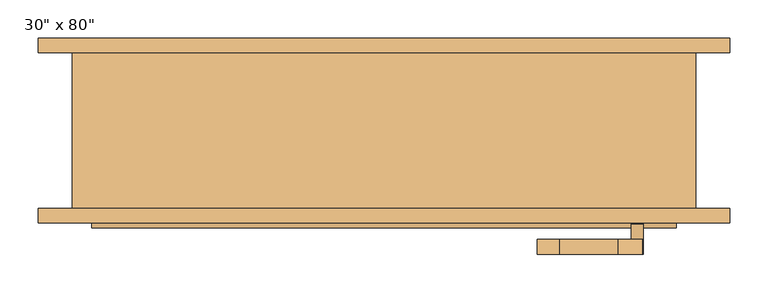
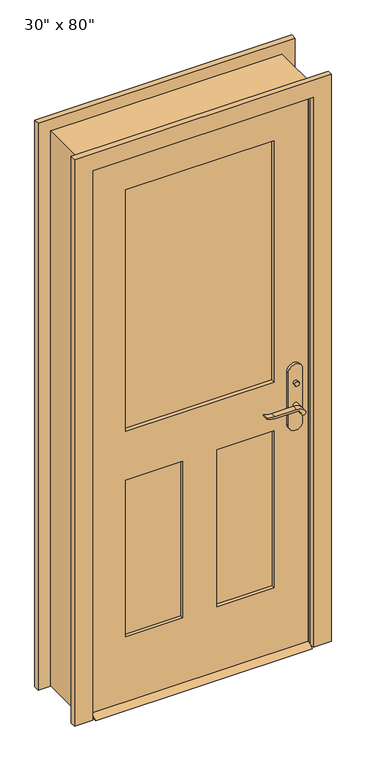
"""IFC4 building model written with IfcOpenShell, lengths in millimetres: door geometry."""

from ifc_helpers import new_model, si_unit, point, frame, frame_2d, origin, place, context, project, spatial, polyline, circle_curve, trimmed, segment, composite_curve, outline, extrude, faceted_brep, source, transform, mapped, element, save


def door_7e6851c9(model_context):
    return source(origin(), model_context, "Body", "SolidModel", [
        extrude(outline(polyline([(-63.5, 12.7), (-38.1, 0.0), (-123.825, 0.0), (-98.425, 12.7), (-63.5, 12.7)])), frame((-381.0, 0.0, 0.0), z_axis=(1.0, 0.0, 0.0), x_axis=(0.0, 1.0, 0.0)), (0.0, 0.0, 1.0), 762.0),
        extrude(outline(polyline([(335.2, -43.5), (335.2, -53.5), (325.2, -53.5), (325.2, -43.5), (335.2, -43.5)])), frame((0.0, 0.0, 981.9), z_axis=(0.0, 0.0, 1.0), x_axis=(1.0, 0.0, 0.0)), (0.0, 0.0, 1.0), 30.0),
        extrude(outline(composite_curve([segment(trimmed(circle_curve(frame_2d((996.9, 330.2)), 8.0), [point((996.9, 322.2))], [point((996.9, 338.2))], False, "CARTESIAN"), True, "CONTINUOUS"), segment(trimmed(circle_curve(frame_2d((996.9, 330.2)), 8.0), [point((996.9, 338.2))], [point((996.9, 322.2))], False, "CARTESIAN"), True, "CONTINUOUS")], self_intersect=False)), frame((0.0, -118.425, 0.0), z_axis=(0.0, 1.0, 0.0), x_axis=(0.0, 0.0, 1.0)), (0.0, 0.0, 1.0), 10.0),
        extrude(outline(composite_curve([segment(trimmed(circle_curve(frame_2d((897.1555521, 306.5324871)), 37.2832219), [point((919.0523287, 336.7081363))], [point((934.4, 304.8325667))], False, "CARTESIAN"), True, "CONTINUOUS"), segment(polyline([(934.4, 304.8325667), (934.4, 228.5564091)]), True, "CONTINUOUS"), segment(trimmed(circle_curve(frame_2d((1017.6850638, 228.6227909)), 83.2850902), [point((934.4, 228.5564091))], [point((939.4, 200.2))], True, "CARTESIAN"), True, "CONTINUOUS"), segment(polyline([(939.4, 200.2), (936.6135558, 200.2)]), True, "CONTINUOUS"), segment(trimmed(circle_curve(frame_2d((986.6709207, 232.1396612)), 59.3791355), [point((936.6135558, 200.2))], [point((927.4, 228.5564091))], False, "CARTESIAN"), True, "CONTINUOUS"), segment(polyline([(927.4, 228.5564091), (927.4, 304.8138099)]), True, "CONTINUOUS"), segment(trimmed(circle_curve(frame_2d((909.2738613, 304.8138099)), 18.1261387), [point((927.4, 304.8138099))], [point((914.4, 322.2))], True, "CARTESIAN"), True, "CONTINUOUS"), segment(trimmed(circle_curve(frame_2d((914.4, 330.2)), 8.0), [point((914.4, 322.2))], [point((919.0523287, 336.7081363))], False, "CARTESIAN"), True, "CONTINUOUS")], self_intersect=False)), frame((0.0, -23.5, 0.0), z_axis=(0.0, 1.0, 0.0), x_axis=(0.0, 0.0, 1.0)), (0.0, 0.0, 1.0), 20.0),
        extrude(outline(composite_curve([segment(trimmed(circle_curve(frame_2d((914.4, 330.2)), 8.0), [point((914.3999903, 322.2))], [point((919.0523287, 336.7081363))], False, "CARTESIAN"), True, "CONTINUOUS"), segment(trimmed(circle_curve(frame_2d((897.1555521, 306.5324871)), 37.2832219), [point((919.0523287, 336.7081363))], [point((934.4, 304.8325667))], False, "CARTESIAN"), True, "CONTINUOUS"), segment(polyline([(934.4, 304.8325667), (934.4, 228.5564091)]), True, "CONTINUOUS"), segment(trimmed(circle_curve(frame_2d((1017.6850638, 228.6227909)), 83.2850902), [point((934.4, 228.5564091))], [point((939.4, 200.2))], True, "CARTESIAN"), True, "CONTINUOUS"), segment(polyline([(939.4, 200.2), (936.6135558, 200.2)]), True, "CONTINUOUS"), segment(trimmed(circle_curve(frame_2d((986.6709207, 232.1396612)), 59.3791355), [point((936.6135558, 200.2))], [point((927.4, 228.5564091))], False, "CARTESIAN"), True, "CONTINUOUS"), segment(polyline([(927.4, 228.5564091), (927.4, 304.8138122)]), True, "CONTINUOUS"), segment(trimmed(circle_curve(frame_2d((909.2738682, 304.8138122)), 18.1261318), [point((927.4, 304.8138122))], [point((914.3999903, 322.2))], True, "CARTESIAN"), True, "CONTINUOUS")], self_intersect=False)), frame((0.0, -158.425, 0.0), z_axis=(0.0, 1.0, 0.0), x_axis=(0.0, 0.0, 1.0)), (0.0, 0.0, 1.0), 20.0),
        extrude(outline(composite_curve([segment(trimmed(circle_curve(frame_2d((914.4, 330.2)), 8.0), [point((914.4, 322.2))], [point((914.4, 338.2))], False, "CARTESIAN"), True, "CONTINUOUS"), segment(trimmed(circle_curve(frame_2d((914.4, 330.2)), 8.0), [point((914.4, 338.2))], [point((914.4, 322.2))], False, "CARTESIAN"), True, "CONTINUOUS")], self_intersect=False)), frame((0.0, -53.5, 0.0), z_axis=(0.0, 1.0, 0.0), x_axis=(0.0, 0.0, 1.0)), (0.0, 0.0, 1.0), 30.0),
        extrude(outline(composite_curve([segment(trimmed(circle_curve(frame_2d((914.4, 330.2)), 8.0), [point((914.4, 322.2))], [point((914.4, 338.2))], False, "CARTESIAN"), True, "CONTINUOUS"), segment(trimmed(circle_curve(frame_2d((914.4, 330.2)), 8.0), [point((914.4, 338.2))], [point((914.4, 322.2))], False, "CARTESIAN"), True, "CONTINUOUS")], self_intersect=False)), frame((0.0, -138.425, 0.0), z_axis=(0.0, 1.0, 0.0), x_axis=(0.0, 0.0, 1.0)), (0.0, 0.0, 1.0), 30.0),
        extrude(outline(composite_curve([segment(polyline([(844.4, 355.2), (1039.4, 355.2)]), True, "CONTINUOUS"), segment(trimmed(circle_curve(frame_2d((1039.4, 330.2)), 25.0), [point((1039.4, 355.2))], [point((1039.4, 305.2))], False, "CARTESIAN"), True, "CONTINUOUS"), segment(polyline([(1039.4, 305.2), (844.4, 305.2)]), True, "CONTINUOUS"), segment(trimmed(circle_curve(frame_2d((844.4, 330.2)), 25.0), [point((844.4, 305.2))], [point((844.4, 355.2))], False, "CARTESIAN"), True, "CONTINUOUS")], self_intersect=False)), frame((0.0, -63.5, 0.0), z_axis=(0.0, 1.0, 0.0), x_axis=(0.0, 0.0, 1.0)), (0.0, 0.0, 1.0), 10.0),
        extrude(outline(composite_curve([segment(polyline([(844.4, 355.2), (1039.4, 355.2)]), True, "CONTINUOUS"), segment(trimmed(circle_curve(frame_2d((1039.4, 330.2)), 25.0), [point((1039.4, 355.2))], [point((1039.4, 305.2))], False, "CARTESIAN"), True, "CONTINUOUS"), segment(polyline([(1039.4, 305.2), (844.4, 305.2)]), True, "CONTINUOUS"), segment(trimmed(circle_curve(frame_2d((844.4, 330.2)), 25.0), [point((844.4, 305.2))], [point((844.4, 355.2))], False, "CARTESIAN"), True, "CONTINUOUS")], self_intersect=False)), frame((0.0, -108.425, 0.0), z_axis=(0.0, 1.0, 0.0), x_axis=(0.0, 0.0, 1.0)), (0.0, 0.0, 1.0), 10.0),
        extrude(outline(polyline([(2032.0, -381.0), (12.7, -381.0), (12.7, 381.0), (2032.0, 381.0), (2032.0, -381.0)]), holes=[polyline([(1016.0, -260.35), (1911.35, -260.35), (1911.35, 260.35), (1016.0, 260.35), (1016.0, -260.35)]), polyline([(835.025, -60.325), (254.0, -60.325), (254.0, -260.35), (835.025, -260.35), (835.025, -60.325)]), polyline([(835.025, 260.35), (254.0, 260.35), (254.0, 60.325), (835.025, 60.325), (835.025, 260.35)])]), frame((0.0, -98.425, 0.0), z_axis=(0.0, 1.0, 0.0), x_axis=(0.0, 0.0, 1.0)), (0.0, 0.0, 1.0), 34.925),
        faceted_brep([(406.4, -98.425, 0.0), (381.0, -98.425, 0.0), (381.0, -63.5, 0.0), (368.3, -63.5, 0.0), (368.3, -28.575, 0.0), (381.0, -28.575, 0.0), (381.0, 104.775, 0.0), (406.4, 104.775, 0.0), (406.4, 104.775, 2057.4), (406.4, -98.425, 2057.4), (381.0, 104.775, 2032.0), (-381.0, 104.775, 2032.0), (-381.0, 104.775, 0.0), (-406.4, 104.775, 0.0), (-406.4, 104.775, 2057.4), (381.0, -28.575, 2032.0), (368.3, -28.575, 2019.3), (-368.3, -28.575, 2019.3), (-368.3, -28.575, 0.0), (-381.0, -28.575, 0.0), (-381.0, -28.575, 2032.0), (368.3, -63.5, 2019.3), (381.0, -63.5, 2032.0), (-381.0, -63.5, 2032.0), (-381.0, -63.5, 0.0), (-368.3, -63.5, 0.0), (-368.3, -63.5, 2019.3), (381.0, -98.425, 2032.0), (-406.4, -98.425, 2057.4), (-406.4, -98.425, 0.0), (-381.0, -98.425, 0.0), (-381.0, -98.425, 2032.0)], [[[0, 1, 2, 3, 4, 5, 6, 7]], [[7, 8, 9, 0]], [[6, 10, 11, 12, 13, 14, 8, 7]], [[5, 15, 10, 6]], [[4, 16, 17, 18, 19, 20, 15, 5]], [[3, 21, 16, 4]], [[2, 22, 23, 24, 25, 26, 21, 3]], [[1, 27, 22, 2]], [[0, 9, 28, 29, 30, 31, 27, 1]], [[8, 14, 28, 9]], [[15, 20, 11, 10]], [[21, 26, 17, 16]], [[27, 31, 23, 22]], [[29, 13, 12, 19, 18, 25, 24, 30]], [[14, 13, 29, 28]], [[20, 19, 12, 11]], [[26, 25, 18, 17]], [[31, 30, 24, 23]]]),
        extrude(outline(polyline([(-60.325, -75.1416667), (-60.325, -86.7833333), (-260.35, -86.7833333), (-260.35, -75.1416667), (-60.325, -75.1416667)])), frame((0.0, 0.0, 254.0), z_axis=(0.0, 0.0, 1.0), x_axis=(1.0, 0.0, 0.0)), (0.0, 0.0, 1.0), 581.025),
        extrude(outline(polyline([(260.35, -75.1416667), (260.35, -86.7833333), (60.325, -86.7833333), (60.325, -75.1416667), (260.35, -75.1416667)])), frame((0.0, 0.0, 254.0), z_axis=(0.0, 0.0, 1.0), x_axis=(1.0, 0.0, 0.0)), (0.0, 0.0, 1.0), 581.025),
        extrude(outline(polyline([(260.35, -77.47), (260.35, -84.455), (-260.35, -84.455), (-260.35, -77.47), (260.35, -77.47)])), frame((0.0, 0.0, 1016.0), z_axis=(0.0, 0.0, 1.0), x_axis=(1.0, 0.0, 0.0)), (0.0, 0.0, 1.0), 895.35),
        extrude(outline(polyline([(0.0, -387.35), (2038.35, -387.35), (2038.35, 387.35), (0.0, 387.35), (0.0, 450.85), (2101.85, 450.85), (2101.85, -450.85), (0.0, -450.85), (0.0, -387.35)])), frame((0.0, 104.775, 0.0), z_axis=(0.0, 1.0, 0.0), x_axis=(0.0, 0.0, 1.0)), (0.0, 0.0, 1.0), 19.05),
        extrude(outline(polyline([(0.0, -387.35), (2038.35, -387.35), (2038.35, 387.35), (0.0, 387.35), (0.0, 450.85), (2101.85, 450.85), (2101.85, -450.85), (0.0, -450.85), (0.0, -387.35)])), frame((0.0, -117.475, 0.0), z_axis=(0.0, 1.0, 0.0), x_axis=(0.0, 0.0, 1.0)), (0.0, 0.0, 1.0), 19.05),
    ])


if __name__ == "__main__":
    model = new_model("IFC4")
    model_context = context("Model", 3, world=origin())
    ifc_project = project(units=[si_unit("LENGTHUNIT", "METRE", prefix="MILLI")], contexts=[model_context])
    site = spatial("IfcSite", under=ifc_project)
    building = spatial("IfcBuilding", under=site)
    placement = place(None, origin())
    door_shape = door_7e6851c9(model_context)
    element("IfcDoor", 1, ObjectType="30\" x 80\"", at=placement, inside=building, context=model_context, shape_type="MappedRepresentation", body=[
        mapped(door_shape, transform((0.0, 0.0, 0.0), x_axis=(1.0, 0.0, 0.0), y_axis=(0.0, 1.0, 0.0), z_axis=(0.0, 0.0, 1.0))),
    ])
    save(model, "model.ifc")

# Revit data of these elements
# Type "30\" x 80\""
#   Type Mark = "8"
#   Assembly Code = "B2030100"
#   Analytic Construction = "French door, wood frame with single glass"
#   Top Rail = 0' - 4 3/4"
#   Threshold Offset [instance default] = 0' - 0 1/2"
#   Thickness = 0' - 1 3/8"
#   Thermal Resistance (R) = 1.0696 (h·ft²·°F)/BTU
#   Swing Angle [instance default] = 90.00°
#   Stiles = 0' - 4 3/4"
#   Rough Width = 2' - 8"
#   Rough Height = 6' - 9"
#   Lock Rail = 0' - 7 1/8"
#   Height = 6' - 8"
#   Width = 2' - 6"
#   Heat Transfer Coefficient (U) = 0.9350 BTU/(h·ft²·°F)
#   Door Offset [instance default] = 0' - 0"
#   Bottom Rail = 0' - 9 1/2"
#   Threshold [instance default] = yes
#   Function = 1
#   Exterior Trim [instance default] = yes
#   Trim Material = Cherry
#   Threshold Material = Cherry
#   Panel Material = Cherry
#   Glazing = Glass
#   Frame Material = Cherry
#   Door Handle Material = Aluminum
#   Visual Light Transmittance = 0
#   Solar Heat Gain Coefficient = 0
#   Wall Closure = (empty or 0)
#   Construction Type = (empty or 0)
# Element 1 (IfcDoor, "30\" x 80\"")
#   Materials on its faces: "Cherry", "Aluminum", "Glass"
# Materials
#   "Cherry": class "Wood", colour RGB 226 177 128, transparency 0, Description = "Prunus Serotina", Cost = 0
#   "Glass": class "Glass", colour RGB 0 128 192, transparency 0.75, Description = "Soda Lime Glass", Cost = 0
#   "Aluminum": class "Metal", colour RGB 247 247 247, transparency 0, Description = "Aluminum 6061", Cost = 0
